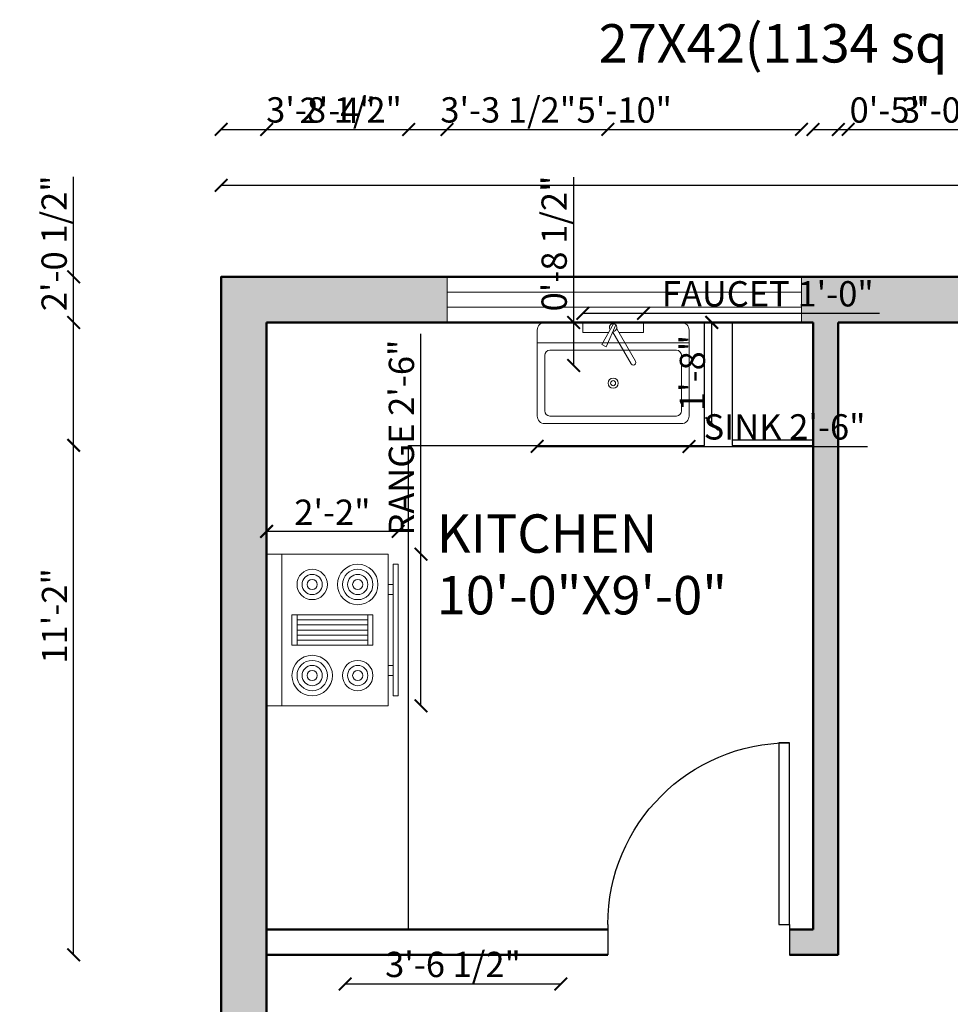
# Model space of a CAD drawing. Units: inches. Extents: x 1799 to 2247, y 1296 to 1881.
# Tile 3 of 4: x 1799 to 1983, y 1687 to 1881. Entities that reach past the tile are written whole.
import ezdxf

# ---------------------------------------------------------------- set-up
doc = ezdxf.new("R2010")
doc.units = ezdxf.units.IN
for name, color, linetype, lineweight in [('A-ANNO-DIMS', 2, 'Continuous', 18), ('A-ANNO-TEXT', 7, 'Continuous', 35), ('A-AREA-IDEN', 7, 'Continuous', 25), ('A-DOOR', 3, 'Continuous', 25), ('A-EQPM', 9, 'Continuous', 18), ('A-FLOR-CASE', 8, 'Continuous', 25), ('A-FLOR-FIXT', 9, 'Continuous', 18), ('A-WALL', 7, 'Continuous', 50), ('window', 4, 'Continuous', 18)]:
    doc.layers.add(name, color=color, linetype=linetype, lineweight=lineweight)
doc.layers.add('A-WALL-PATT', color=18, linetype='Continuous', lineweight=13, true_color=0x000000)
doc.styles.get("Standard").update_dxf_attribs({"font": 'arial.ttf'})
doc.dimstyles.new('ISO-25', dxfattribs={"dimtxt": 5, "dimasz": 2.5, "dimexe": 1.25, "dimexo": 0.625, "dimtad": 1, "dimdec": 0, "dimlunit": 4, "dimtxsty": 'Standard', "dimblk": 'ARCHTICK', "dimcen": 2.5, "dimse1": 1, "dimse2": 1, "dimclrd": 1, "dimadec": 0, "dimazin": 0, "dimtfac": 1, "dimtdec": 0, "dimtmove": 0, "dimatfit": 3, "dimfxl": 1, "dimarcsym": 0})

# ---------------------------------------------------------------- blocks, each defined once
blk = doc.blocks.new('Range-Oven - 30 in top')
for p, q in [((0, -3), (30, -3)), ((12, -6), (18, -6)), ((13, -20), (13, -6)), ((14, -6), (14, -20)), ((15, -20), (15, -6)), ((16, -6), (16, -20)), ((17, -20), (17, -6)), ((18, -20), (12, -20)), ((6, -24), (6, -25)), ((8, -25), (8, -24)), ((22, -25), (22, -24)), ((24, -24), (24, -25))]:
    blk.add_line(p, q)
for points in [[(0, -24), (0, 0), (30, 0), (30, -24)], [(12, -21), (12, -5), (18, -5), (18, -21)], [(2, -26), (2, -25), (28, -25), (28, -26)]]:
    blk.add_lwpolyline(points, close=True)
for centre, radius in [((6, -9), 4), ((6, -9), 3), ((6, -9), 2), ((24, -9), 3), ((24, -9), 2), ((6, -9), 1), ((24, -9), 1), ((6, -18), 3), ((24, -18), 4), ((24, -18), 3), ((6, -18), 2), ((6, -18), 1), ((24, -18), 2), ((24, -18), 1)]:
    blk.add_circle(centre, radius)
blk = doc.blocks.new('Faucet - single handle top')
for p, q in [((0.08, -0.26), (-2.26, -4.34)), ((-1.37, -4.79), (0.55, -0.5)), ((-0.06, -1.9), (3.57, -8.18)), ((4.43, -7.68), (0.72, -1.24)), ((-2.26, -4.34), (-1.37, -4.79))]:
    blk.add_line(p, q)
for points in [[(-0.92, -2), (-6, -2), (-6, 0), (6, 0), (6, -2), (1.16, -2)], [(-0.01, -2), (-0.12, -2)]]:
    blk.add_lwpolyline(points)
for centre, radius, start, end in [((0, -1), 0.75, 269.2246, 216.2304), ((4, -7.93), 0.5, 210, 30)]:
    blk.add_arc(centre, radius, start, end)
blk = doc.blocks.new('*U12')
for p, q in [((0, 0), (0, -5)), ((30, 0), (30, -5))]:
    blk.add_line(p, q)
blk.add_lwpolyline([(0, 0), (0, 30), (1.75, 30), (1.75, 0)], close=True)
blk.add_arc((0, 0), 30, 0, 90)
blk = doc.blocks.new('Sink-single - 30 in top')
blk.add_line((-15, -3.999996), (15, -3.999996))
for points in [[(-13.5, 0), (13.5, 0)], [(-15, -18.499996), (-15, -1.5)], [(15, -1.5), (15, -18.499996)], [(-12.5, -5.499996), (12.5, -5.499996)], [(-13.5, -17.499996), (-13.5, -6.499996)], [(13.5, -6.499996), (13.5, -17.499996)], [(12.5, -18.499996), (-12.5, -18.499996)], [(13.5, -19.999996), (-13.5, -19.999996)]]:
    blk.add_lwpolyline(points)
for radius in [1, 0.5]:
    blk.add_circle((0, -11.999996), radius)
for centre, radius, start, end in [((-13.5, -1.5), 1.5, 90, 180), ((13.5, -1.5), 1.5, 0, 90), ((-12.5, -6.499996), 1, 90, 180), ((12.5, -6.499996), 1, 0, 90), ((-12.5, -17.499996), 1, 180, 270), ((12.5, -17.499996), 1, 270, 0), ((-13.5, -18.499996), 1.5, 180, 270), ((13.5, -18.499996), 1.5, 270, 0)]:
    blk.add_arc(centre, radius, start, end)
blk = doc.blocks.new('_ArchTick')
at = {"color": 0, "linetype": 'ByBlock', "const_width": 0.15}
blk.add_lwpolyline([(-0.5, -0.5), (0.5, 0.5)], dxfattribs=at)
blk = doc.blocks.new('*D13')
at = {"layer": 'A-ANNO-DIMS', "color": 0, "lineweight": -2, "transparency": 16777216}
blk.add_line((1838.46, 1848.42), (2162.46, 1848.42), dxfattribs=at)
at = {"layer": 'Defpoints', "color": 0, "transparency": 16777216}
for p in [(2162.46, 1848.42), (1838.46, 1830.32), (2162.46, 1830.32)]:
    blk.add_point(p, dxfattribs=at)
at = {"layer": 'A-ANNO-DIMS', "color": 0, "lineweight": -2, "transparency": 16777216, "xscale": 2.5, "yscale": 2.5, "zscale": 2.5, "rotation": 180}
blk.add_blockref('_ArchTick', (1838.46, 1848.42), dxfattribs=at)
at = {"layer": 'A-ANNO-DIMS', "color": 0, "lineweight": -2, "transparency": 16777216, "xscale": 2.5, "yscale": 2.5, "zscale": 2.5}
blk.add_blockref('_ArchTick', (2162.46, 1848.42), dxfattribs=at)
at = {"layer": 'A-ANNO-DIMS', "color": 0, "transparency": 16777216, "insert": (2000.46, 1851.56), "char_height": 5, "attachment_point": 5}
blk.add_mtext("27'", dxfattribs=at)
blk = doc.blocks.new('*D23')
at = {"layer": 'A-ANNO-DIMS', "color": 1, "lineweight": -2, "transparency": 16777216}
blk.add_line((1862.99, 1690.58), (1905.61, 1690.58), dxfattribs=at)
at = {"layer": 'Defpoints', "color": 0, "transparency": 16777216}
for p in [(1905.61, 1690.58), (1862.99, 1680), (1905.61, 1680)]:
    blk.add_point(p, dxfattribs=at)
at = {"layer": 'A-ANNO-DIMS', "color": 1, "lineweight": -2, "transparency": 16777216, "xscale": 2.5, "yscale": 2.5, "zscale": 2.5, "rotation": 180}
blk.add_blockref('_ArchTick', (1862.99, 1690.58), dxfattribs=at)
at = {"layer": 'A-ANNO-DIMS', "color": 1, "lineweight": -2, "transparency": 16777216, "xscale": 2.5, "yscale": 2.5, "zscale": 2.5}
blk.add_blockref('_ArchTick', (1905.61, 1690.58), dxfattribs=at)
at = {"layer": 'A-ANNO-DIMS', "color": 0, "transparency": 16777216, "insert": (1884.3, 1693.79), "char_height": 5, "attachment_point": 5}
blk.add_mtext('3\'-6 1/2"', dxfattribs=at)
blk = doc.blocks.new('*D24')
at = {"layer": 'A-ANNO-DIMS', "color": 1, "lineweight": -2, "transparency": 16777216}
for p, q in [((1877.96, 1775.53), (1877.96, 1819.09)), ((1877.96, 1745.53), (1877.96, 1775.53))]:
    blk.add_line(p, q, dxfattribs=at)
at = {"layer": 'Defpoints', "color": 0, "transparency": 16777216}
for p in [(1873.46, 1775.53), (1877.96, 1775.53), (1873.46, 1745.53)]:
    blk.add_point(p, dxfattribs=at)
at = {"layer": 'A-ANNO-DIMS', "color": 1, "lineweight": -2, "transparency": 16777216, "xscale": 2.5, "yscale": 2.5, "zscale": 2.5}
for p, rotation in [((1877.96, 1775.53), 90), ((1877.96, 1745.53), 270)]:
    blk.add_blockref('_ArchTick', p, dxfattribs=dict(at, rotation=rotation))
at = {"layer": 'A-ANNO-DIMS', "color": 0, "transparency": 16777216, "insert": (1874.75, 1798.56), "char_height": 5, "attachment_point": 5, "rotation": 90}
blk.add_mtext('RANGE 2\'-6"', dxfattribs=at)
blk = doc.blocks.new('*D25')
at = {"layer": 'A-ANNO-DIMS', "color": 1, "lineweight": -2, "transparency": 16777216}
blk.add_line((1873.46, 1780.03), (1847.46, 1780.03), dxfattribs=at)
at = {"layer": 'Defpoints', "color": 0, "transparency": 16777216}
for p in [(1847.46, 1780.03), (1847.46, 1775.53), (1873.46, 1775.53)]:
    blk.add_point(p, dxfattribs=at)
at = {"layer": 'A-ANNO-DIMS', "color": 1, "lineweight": -2, "transparency": 16777216, "xscale": 2.5, "yscale": 2.5, "zscale": 2.5, "rotation": 180}
blk.add_blockref('_ArchTick', (1847.46, 1780.03), dxfattribs=at)
at = {"layer": 'A-ANNO-DIMS', "color": 1, "lineweight": -2, "transparency": 16777216, "xscale": 2.5, "yscale": 2.5, "zscale": 2.5}
blk.add_blockref('_ArchTick', (1873.46, 1780.03), dxfattribs=at)
at = {"layer": 'A-ANNO-DIMS', "color": 0, "transparency": 16777216, "insert": (1860.46, 1783.16), "char_height": 5, "attachment_point": 5}
blk.add_mtext('2\'-2"', dxfattribs=at)
blk = doc.blocks.new('*D26')
at = {"layer": 'A-ANNO-DIMS', "color": 1, "lineweight": -2, "transparency": 16777216}
for p, q in [((1900.95, 1796.82), (1930.95, 1796.82)), ((1930.95, 1796.82), (1966.21, 1796.82))]:
    blk.add_line(p, q, dxfattribs=at)
at = {"layer": 'Defpoints', "color": 0, "transparency": 16777216}
for p in [(1900.95, 1801.32), (1930.95, 1801.32), (1930.95, 1796.82)]:
    blk.add_point(p, dxfattribs=at)
at = {"layer": 'A-ANNO-DIMS', "color": 1, "lineweight": -2, "transparency": 16777216, "xscale": 2.5, "yscale": 2.5, "zscale": 2.5, "rotation": 180}
blk.add_blockref('_ArchTick', (1900.95, 1796.82), dxfattribs=at)
at = {"layer": 'A-ANNO-DIMS', "color": 1, "lineweight": -2, "transparency": 16777216, "xscale": 2.5, "yscale": 2.5, "zscale": 2.5}
blk.add_blockref('_ArchTick', (1930.95, 1796.82), dxfattribs=at)
at = {"layer": 'A-ANNO-DIMS', "color": 0, "transparency": 16777216, "insert": (1949.83, 1800.03), "char_height": 5, "attachment_point": 5}
blk.add_mtext('SINK 2\'-6"', dxfattribs=at)
blk = doc.blocks.new('*D27')
at = {"layer": 'A-ANNO-DIMS', "color": 1, "lineweight": -2, "transparency": 16777216}
blk.add_line((1935.45, 1801.32), (1935.45, 1821.32), dxfattribs=at)
at = {"layer": 'Defpoints', "color": 0, "transparency": 16777216}
for p in [(1930.95, 1821.32), (1935.45, 1821.32), (1930.95, 1801.32)]:
    blk.add_point(p, dxfattribs=at)
at = {"layer": 'A-ANNO-DIMS', "color": 1, "lineweight": -2, "transparency": 16777216, "xscale": 2.5, "yscale": 2.5, "zscale": 2.5}
for p, rotation in [((1935.45, 1821.32), 90), ((1935.45, 1801.32), 270)]:
    blk.add_blockref('_ArchTick', p, dxfattribs=dict(at, rotation=rotation))
at = {"layer": 'A-ANNO-DIMS', "color": 0, "transparency": 16777216, "insert": (1932.27, 1811.32), "char_height": 5, "attachment_point": 5, "rotation": 90}
blk.add_mtext('1\'-8"', dxfattribs=at)
blk = doc.blocks.new('*D28')
at = {"layer": 'A-ANNO-DIMS', "color": 1, "lineweight": -2, "transparency": 16777216}
for p, q in [((1909.95, 1823.12), (1921.95, 1823.12)), ((1921.95, 1823.12), (1968.59, 1823.12))]:
    blk.add_line(p, q, dxfattribs=at)
at = {"layer": 'Defpoints', "color": 0, "transparency": 16777216}
for p in [(1921.95, 1823.12), (1909.95, 1821.32), (1921.95, 1821.32)]:
    blk.add_point(p, dxfattribs=at)
at = {"layer": 'A-ANNO-DIMS', "color": 1, "lineweight": -2, "transparency": 16777216, "xscale": 2.5, "yscale": 2.5, "zscale": 2.5, "rotation": 180}
blk.add_blockref('_ArchTick', (1909.95, 1823.12), dxfattribs=at)
at = {"layer": 'A-ANNO-DIMS', "color": 1, "lineweight": -2, "transparency": 16777216, "xscale": 2.5, "yscale": 2.5, "zscale": 2.5}
blk.add_blockref('_ArchTick', (1921.95, 1823.12), dxfattribs=at)
at = {"layer": 'A-ANNO-DIMS', "color": 0, "transparency": 16777216, "insert": (1946.52, 1826.33), "char_height": 5, "attachment_point": 5}
blk.add_mtext('FAUCET 1\'-0"', dxfattribs=at)
blk = doc.blocks.new('*D29')
at = {"layer": 'A-ANNO-DIMS', "color": 1, "lineweight": -2, "transparency": 16777216}
for p, q in [((1908.15, 1821.32), (1908.15, 1850.01)), ((1908.15, 1812.82), (1908.15, 1821.32))]:
    blk.add_line(p, q, dxfattribs=at)
at = {"layer": 'Defpoints', "color": 0, "transparency": 16777216}
for p in [(1908.15, 1821.32), (1909.95, 1821.32), (1909.95, 1812.82)]:
    blk.add_point(p, dxfattribs=at)
at = {"layer": 'A-ANNO-DIMS', "color": 1, "lineweight": -2, "transparency": 16777216, "xscale": 2.5, "yscale": 2.5, "zscale": 2.5}
for p, rotation in [((1908.15, 1821.32), 90), ((1908.15, 1812.82), 270)]:
    blk.add_blockref('_ArchTick', p, dxfattribs=dict(at, rotation=rotation))
at = {"layer": 'A-ANNO-DIMS', "color": 0, "transparency": 16777216, "insert": (1904.94, 1836.92), "char_height": 5, "attachment_point": 5, "rotation": 90}
blk.add_mtext('0\'-8 1/2"', dxfattribs=at)
blk = doc.blocks.new('*D34')
at = {"layer": 'A-ANNO-DIMS', "color": 1, "lineweight": -2, "transparency": 16777216}
blk.add_line((1809.31, 1696.32), (1809.31, 1830.32), dxfattribs=at)
at = {"layer": 'Defpoints', "color": 0, "transparency": 16777216}
for p in [(1809.31, 1830.32), (1838.46, 1830.32), (1847.46, 1696.32)]:
    blk.add_point(p, dxfattribs=at)
at = {"layer": 'A-ANNO-DIMS', "color": 1, "lineweight": -2, "transparency": 16777216, "xscale": 2.5, "yscale": 2.5, "zscale": 2.5}
for p, rotation in [((1809.31, 1830.32), 90), ((1809.31, 1696.32), 270)]:
    blk.add_blockref('_ArchTick', p, dxfattribs=dict(at, rotation=rotation))
at = {"layer": 'A-ANNO-DIMS', "color": 0, "transparency": 16777216, "insert": (1806.17, 1763.32), "char_height": 5, "attachment_point": 5, "rotation": 90}
blk.add_mtext('11\'-2"', dxfattribs=at)
blk = doc.blocks.new('*D35')
at = {"layer": 'A-ANNO-DIMS', "color": 1, "lineweight": -2, "transparency": 16777216}
blk.add_line((1960.46, 1297.17), (2076.46, 1297.17), dxfattribs=at)
at = {"layer": 'Defpoints', "color": 0, "transparency": 16777216}
for p in [(1960.46, 1821.32), (2076.46, 1821.32), (2076.46, 1297.17)]:
    blk.add_point(p, dxfattribs=at)
at = {"layer": 'A-ANNO-DIMS', "color": 1, "lineweight": -2, "transparency": 16777216, "xscale": 2.5, "yscale": 2.5, "zscale": 2.5, "rotation": 180}
blk.add_blockref('_ArchTick', (1960.46, 1297.17), dxfattribs=at)
at = {"layer": 'A-ANNO-DIMS', "color": 1, "lineweight": -2, "transparency": 16777216, "xscale": 2.5, "yscale": 2.5, "zscale": 2.5}
blk.add_blockref('_ArchTick', (2076.46, 1297.17), dxfattribs=at)
at = {"layer": 'A-ANNO-DIMS', "color": 0, "transparency": 16777216, "insert": (2018.46, 1300.35), "char_height": 5, "attachment_point": 5}
blk.add_mtext('9\'-8"', dxfattribs=at)
blk = doc.blocks.new('*D36')
at = {"layer": 'A-ANNO-DIMS', "color": 1, "lineweight": -2, "transparency": 16777216}
blk.add_line((1847.46, 1859.47), (1875.53, 1859.47), dxfattribs=at)
at = {"layer": 'Defpoints', "color": 0, "transparency": 16777216}
for p in [(1875.53, 1859.47), (1847.46, 1701.32), (1875.53, 1701.32)]:
    blk.add_point(p, dxfattribs=at)
at = {"layer": 'A-ANNO-DIMS', "color": 1, "lineweight": -2, "transparency": 16777216, "xscale": 2.5, "yscale": 2.5, "zscale": 2.5, "rotation": 180}
blk.add_blockref('_ArchTick', (1847.46, 1859.47), dxfattribs=at)
at = {"layer": 'A-ANNO-DIMS', "color": 1, "lineweight": -2, "transparency": 16777216, "xscale": 2.5, "yscale": 2.5, "zscale": 2.5}
blk.add_blockref('_ArchTick', (1875.53, 1859.47), dxfattribs=at)
at = {"layer": 'A-ANNO-DIMS', "color": 0, "transparency": 16777216, "insert": (1861.5, 1862.6), "char_height": 5, "attachment_point": 5}
blk.add_mtext('2\'-4"', dxfattribs=at)
blk = doc.blocks.new('*D45')
at = {"layer": 'A-ANNO-DIMS', "color": 1, "lineweight": -2, "transparency": 16777216}
blk.add_line((1838.46, 1859.47), (1883.11, 1859.47), dxfattribs=at)
at = {"layer": 'Defpoints', "color": 0, "transparency": 16777216}
for p in [(1883.11, 1859.47), (1838.46, 1830.32), (1883.11, 1830.32)]:
    blk.add_point(p, dxfattribs=at)
at = {"layer": 'A-ANNO-DIMS', "color": 1, "lineweight": -2, "transparency": 16777216, "xscale": 2.5, "yscale": 2.5, "zscale": 2.5, "rotation": 180}
blk.add_blockref('_ArchTick', (1838.46, 1859.47), dxfattribs=at)
at = {"layer": 'A-ANNO-DIMS', "color": 1, "lineweight": -2, "transparency": 16777216, "xscale": 2.5, "yscale": 2.5, "zscale": 2.5}
blk.add_blockref('_ArchTick', (1883.11, 1859.47), dxfattribs=at)
at = {"layer": 'A-ANNO-DIMS', "color": 0, "transparency": 16777216, "insert": (1860.78, 1862.68), "char_height": 5, "attachment_point": 5}
blk.add_mtext('3\'-8 1/2"', dxfattribs=at)
blk = doc.blocks.new('*D46')
at = {"layer": 'A-ANNO-DIMS', "color": 1, "lineweight": -2, "transparency": 16777216}
blk.add_line((1883.11, 1859.47), (1953.2, 1859.47), dxfattribs=at)
at = {"layer": 'Defpoints', "color": 0, "transparency": 16777216}
for p in [(1953.2, 1859.47), (1883.11, 1830.32), (1953.2, 1830.32)]:
    blk.add_point(p, dxfattribs=at)
at = {"layer": 'A-ANNO-DIMS', "color": 1, "lineweight": -2, "transparency": 16777216, "xscale": 2.5, "yscale": 2.5, "zscale": 2.5, "rotation": 180}
blk.add_blockref('_ArchTick', (1883.11, 1859.47), dxfattribs=at)
at = {"layer": 'A-ANNO-DIMS', "color": 1, "lineweight": -2, "transparency": 16777216, "xscale": 2.5, "yscale": 2.5, "zscale": 2.5}
blk.add_blockref('_ArchTick', (1953.2, 1859.47), dxfattribs=at)
at = {"layer": 'A-ANNO-DIMS', "color": 0, "transparency": 16777216, "insert": (1918.16, 1862.65), "char_height": 5, "attachment_point": 5}
blk.add_mtext('5\'-10"', dxfattribs=at)
blk = doc.blocks.new('*D47')
at = {"layer": 'A-ANNO-DIMS', "color": 1, "lineweight": -2, "transparency": 16777216}
blk.add_line((1914.89, 1297.17), (1950.83, 1297.17), dxfattribs=at)
at = {"layer": 'Defpoints', "color": 0, "transparency": 16777216}
for p in [(1914.89, 1701.32), (1950.83, 1701.32), (1950.83, 1297.17)]:
    blk.add_point(p, dxfattribs=at)
at = {"layer": 'A-ANNO-DIMS', "color": 1, "lineweight": -2, "transparency": 16777216, "xscale": 2.5, "yscale": 2.5, "zscale": 2.5, "rotation": 180}
blk.add_blockref('_ArchTick', (1914.89, 1297.17), dxfattribs=at)
at = {"layer": 'A-ANNO-DIMS', "color": 1, "lineweight": -2, "transparency": 16777216, "xscale": 2.5, "yscale": 2.5, "zscale": 2.5}
blk.add_blockref('_ArchTick', (1950.83, 1297.17), dxfattribs=at)
at = {"layer": 'A-ANNO-DIMS', "color": 0, "transparency": 16777216, "insert": (1932.86, 1300.35), "char_height": 5, "attachment_point": 5}
blk.add_mtext('3\'-0"', dxfattribs=at)
blk = doc.blocks.new('*D48')
at = {"layer": 'A-ANNO-DIMS', "color": 1, "lineweight": -2, "transparency": 16777216}
blk.add_line((1962.42, 1859.47), (1998.36, 1859.47), dxfattribs=at)
at = {"layer": 'Defpoints', "color": 0, "transparency": 16777216}
for p in [(1998.36, 1859.47), (1962.42, 1353.51), (1998.36, 1353.51)]:
    blk.add_point(p, dxfattribs=at)
at = {"layer": 'A-ANNO-DIMS', "color": 1, "lineweight": -2, "transparency": 16777216, "xscale": 2.5, "yscale": 2.5, "zscale": 2.5, "rotation": 180}
blk.add_blockref('_ArchTick', (1962.42, 1859.47), dxfattribs=at)
at = {"layer": 'A-ANNO-DIMS', "color": 1, "lineweight": -2, "transparency": 16777216, "xscale": 2.5, "yscale": 2.5, "zscale": 2.5}
blk.add_blockref('_ArchTick', (1998.36, 1859.47), dxfattribs=at)
at = {"layer": 'A-ANNO-DIMS', "color": 0, "transparency": 16777216, "insert": (1980.39, 1862.65), "char_height": 5, "attachment_point": 5}
blk.add_mtext('3\'-0"', dxfattribs=at)
blk = doc.blocks.new('*D55')
at = {"layer": 'A-ANNO-DIMS', "color": 1, "lineweight": -2, "transparency": 16777216}
blk.add_line((2242.61, 1701.32), (2242.61, 1745.53), dxfattribs=at)
at = {"layer": 'Defpoints', "color": 0, "transparency": 16777216}
for p in [(1847.46, 1745.53), (2242.61, 1745.53), (1847.46, 1701.32)]:
    blk.add_point(p, dxfattribs=at)
at = {"layer": 'A-ANNO-DIMS', "color": 1, "lineweight": -2, "transparency": 16777216, "xscale": 2.5, "yscale": 2.5, "zscale": 2.5}
for p, rotation in [((2242.61, 1745.53), 90), ((2242.61, 1701.32), 270)]:
    blk.add_blockref('_ArchTick', p, dxfattribs=dict(at, rotation=rotation))
at = {"layer": 'A-ANNO-DIMS', "color": 0, "transparency": 16777216, "insert": (2239.43, 1723.42), "char_height": 5, "attachment_point": 5, "rotation": 90}
blk.add_mtext('3\'-8"', dxfattribs=at)
blk = doc.blocks.new('*D56')
at = {"layer": 'A-ANNO-DIMS', "color": 1, "lineweight": -2, "transparency": 16777216}
for p, q in [((1809.31, 1821.32), (1809.31, 1850.1)), ((1809.31, 1797.03), (1809.31, 1821.32))]:
    blk.add_line(p, q, dxfattribs=at)
at = {"layer": 'Defpoints', "color": 0, "transparency": 16777216}
for p in [(1809.31, 1821.32), (1955.46, 1821.32), (1955.46, 1797.03)]:
    blk.add_point(p, dxfattribs=at)
at = {"layer": 'A-ANNO-DIMS', "color": 1, "lineweight": -2, "transparency": 16777216, "xscale": 2.5, "yscale": 2.5, "zscale": 2.5}
for p, rotation in [((1809.31, 1821.32), 90), ((1809.31, 1797.03), 270)]:
    blk.add_blockref('_ArchTick', p, dxfattribs=dict(at, rotation=rotation))
at = {"layer": 'A-ANNO-DIMS', "color": 0, "transparency": 16777216, "insert": (1806.1, 1836.96), "char_height": 5, "attachment_point": 5, "rotation": 90}
blk.add_mtext('2\'-0 1/2"', dxfattribs=at)
blk = doc.blocks.new('*D57')
at = {"layer": 'A-ANNO-DIMS', "color": 1, "lineweight": -2, "transparency": 16777216}
blk.add_line((1875.53, 1297.17), (1901.39, 1297.17), dxfattribs=at)
at = {"layer": 'Defpoints', "color": 0, "transparency": 16777216}
for p in [(1901.39, 1801.76), (1875.53, 1797.03), (1901.39, 1297.17)]:
    blk.add_point(p, dxfattribs=at)
at = {"layer": 'A-ANNO-DIMS', "color": 1, "lineweight": -2, "transparency": 16777216, "xscale": 2.5, "yscale": 2.5, "zscale": 2.5, "rotation": 180}
blk.add_blockref('_ArchTick', (1875.53, 1297.17), dxfattribs=at)
at = {"layer": 'A-ANNO-DIMS', "color": 1, "lineweight": -2, "transparency": 16777216, "xscale": 2.5, "yscale": 2.5, "zscale": 2.5}
blk.add_blockref('_ArchTick', (1901.39, 1297.17), dxfattribs=at)
at = {"layer": 'A-ANNO-DIMS', "color": 0, "transparency": 16777216, "insert": (1888.46, 1300.3), "char_height": 5, "attachment_point": 5}
blk.add_mtext('2\'-2"', dxfattribs=at)
blk = doc.blocks.new('*D61')
at = {"layer": 'A-ANNO-DIMS', "color": 1, "lineweight": -2, "transparency": 16777216}
for p, q in [((1838.46, 1297.17), (1847.46, 1297.17)), ((1847.46, 1297.17), (1864.5, 1297.17))]:
    blk.add_line(p, q, dxfattribs=at)
at = {"layer": 'Defpoints', "color": 0, "transparency": 16777216}
for p in [(1838.46, 1830.32), (1847.46, 1821.32), (1847.46, 1297.17)]:
    blk.add_point(p, dxfattribs=at)
at = {"layer": 'A-ANNO-DIMS', "color": 1, "lineweight": -2, "transparency": 16777216, "xscale": 2.5, "yscale": 2.5, "zscale": 2.5, "rotation": 180}
blk.add_blockref('_ArchTick', (1838.46, 1297.17), dxfattribs=at)
at = {"layer": 'A-ANNO-DIMS', "color": 1, "lineweight": -2, "transparency": 16777216, "xscale": 2.5, "yscale": 2.5, "zscale": 2.5}
blk.add_blockref('_ArchTick', (1847.46, 1297.17), dxfattribs=at)
at = {"layer": 'A-ANNO-DIMS', "color": 0, "transparency": 16777216, "insert": (1857.23, 1300.35), "char_height": 5, "attachment_point": 5}
blk.add_mtext('0\'-9"', dxfattribs=at)
blk = doc.blocks.new('*D62')
at = {"layer": 'A-ANNO-DIMS', "color": 1, "lineweight": -2, "transparency": 16777216}
for p, q in [((1955.46, 1859.47), (1960.46, 1859.47)), ((1960.46, 1859.47), (1977.5, 1859.47))]:
    blk.add_line(p, q, dxfattribs=at)
at = {"layer": 'Defpoints', "color": 0, "transparency": 16777216}
for p in [(1960.46, 1859.47), (1955.46, 1821.32), (1960.46, 1821.32)]:
    blk.add_point(p, dxfattribs=at)
at = {"layer": 'A-ANNO-DIMS', "color": 1, "lineweight": -2, "transparency": 16777216, "xscale": 2.5, "yscale": 2.5, "zscale": 2.5, "rotation": 180}
blk.add_blockref('_ArchTick', (1955.46, 1859.47), dxfattribs=at)
at = {"layer": 'A-ANNO-DIMS', "color": 1, "lineweight": -2, "transparency": 16777216, "xscale": 2.5, "yscale": 2.5, "zscale": 2.5}
blk.add_blockref('_ArchTick', (1960.46, 1859.47), dxfattribs=at)
at = {"layer": 'A-ANNO-DIMS', "color": 0, "transparency": 16777216, "insert": (1970.23, 1862.65), "char_height": 5, "attachment_point": 5}
blk.add_mtext('0\'-5"', dxfattribs=at)
blk = doc.blocks.new('*D63')
at = {"layer": 'A-ANNO-DIMS', "color": 1, "lineweight": -2, "transparency": 16777216}
blk.add_line((1875.53, 1859.47), (1914.89, 1859.47), dxfattribs=at)
at = {"layer": 'Defpoints', "color": 0, "transparency": 16777216}
for p in [(1914.89, 1859.47), (1875.53, 1701.32), (1914.89, 1701.32)]:
    blk.add_point(p, dxfattribs=at)
at = {"layer": 'A-ANNO-DIMS', "color": 1, "lineweight": -2, "transparency": 16777216, "xscale": 2.5, "yscale": 2.5, "zscale": 2.5, "rotation": 180}
blk.add_blockref('_ArchTick', (1875.53, 1859.47), dxfattribs=at)
at = {"layer": 'A-ANNO-DIMS', "color": 1, "lineweight": -2, "transparency": 16777216, "xscale": 2.5, "yscale": 2.5, "zscale": 2.5}
blk.add_blockref('_ArchTick', (1914.89, 1859.47), dxfattribs=at)
at = {"layer": 'A-ANNO-DIMS', "color": 0, "transparency": 16777216, "insert": (1895.21, 1862.68), "char_height": 5, "attachment_point": 5}
blk.add_mtext('3\'-3 1/2"', dxfattribs=at)

msp = doc.modelspace()

# ---------------------------------------------------------------- hatches: boundary and pattern name
at = {"layer": 'A-WALL-PATT'}
h = msp.add_hatch(color=256, dxfattribs=at)
h.dxf.hatch_style = 1
h.paths.add_polyline_path([(1847.46, 1821.32), (1883.11, 1821.32), (1883.11, 1830.32), (1838.46, 1830.32), (1838.46, 1618.8), (1847.46, 1618.8)])
h.paths.add_polyline_path([(1847.46, 1534.31), (1838.46, 1534.31), (1838.46, 1444.97), (1847.46, 1444.97)])
h.paths.add_polyline_path([(1847.46, 1404.13), (1838.46, 1404.13), (1838.46, 1353.51), (1847.46, 1353.51), (1962.42, 1353.51), (1962.42, 1359.5, -0.020971), (1962.55, 1362.51), (1847.46, 1362.51)])
h.paths.add_polyline_path([(2162.46, 1509.73), (2153.46, 1509.73), (2153.46, 1493.32), (2075.46, 1493.32), (2075.46, 1496.56), (2075.02, 1496.56), (2070.46, 1496.56), (2070.46, 1488.32), (2153.46, 1488.32), (2153.46, 1335.32), (2119.37, 1335.32), (2119.37, 1326.32), (2162.46, 1326.32)])
h.paths.add_polyline_path([(2059.58, 1335.32), (2008.46, 1335.32), (2008.46, 1353.51), (2003.46, 1353.51), (2003.46, 1335.32), (2003.46, 1326.32), (2059.58, 1326.32)])
h.paths.add_polyline_path([(2008.46, 1471.58), (2003.46, 1471.58), (2003.46, 1460.32), (1847.46, 1460.32), (1847.46, 1455.32), (2003.46, 1455.32), (2003.46, 1362.51), (2008.46, 1362.51)])
h.paths.add_polyline_path([(2008.46, 1362.51), (2003.46, 1362.51), (2003.46, 1353.51), (2008.46, 1353.51)])
h.paths.add_polyline_path([(2003.46, 1362.51), (1998.36, 1362.51), (1998.36, 1359.5), (1998.36, 1353.51), (2003.46, 1353.51)])
h.paths.add_polyline_path([(1989.49, 1830.32), (1953.2, 1830.32), (1953.2, 1821.32), (1955.46, 1821.32), (1955.46, 1701.32), (1950.83, 1701.32), (1950.83, 1696.32), (1960.46, 1696.32), (1960.46, 1821.32), (1989.49, 1821.32)])
h.paths.add_polyline_path([(2162.46, 1606.83), (2153.46, 1606.83), (2153.46, 1541.93), (2162.46, 1541.93)])
h.paths.add_polyline_path([(2162.46, 1746.71), (2153.46, 1746.71), (2153.46, 1701.32), (2081.46, 1701.32), (2081.46, 1707.91), (2081.05, 1707.91), (2076.46, 1707.91), (2076.46, 1701.32), (2003.46, 1701.32), (2003.46, 1604.81), (2008.46, 1604.81), (2008.46, 1696.32), (2153.46, 1696.32), (2153.46, 1656.83), (2162.46, 1656.83)])
h.paths.add_polyline_path([(2162.46, 1830.32), (2050.89, 1830.32), (2050.89, 1821.32), (2076.46, 1821.32), (2076.46, 1735.44), (2081.05, 1735.44, -0.003736), (2081.46, 1735.44), (2081.46, 1821.32), (2153.46, 1821.32), (2153.46, 1778.8), (2162.46, 1778.8)])
h.paths.add_polyline_path([(1961.29, 1344.27), (2000.99, 1344.27), (2000.99, 1355.65), (1961.29, 1355.65)], flags=9)
h.paths.add_polyline_path([(1882.83, 1491.06), (1947.74, 1491.06), (1947.74, 1502.69), (1882.83, 1502.69)], flags=9)
h.paths.add_polyline_path([(1882.8, 1503.23), (1950.9, 1503.23), (1950.9, 1514.99), (1882.8, 1514.99)], flags=9)
h.paths.add_polyline_path([(2045.91, 1444.14), (2110.82, 1444.14), (2110.82, 1455.75), (2045.91, 1455.75)], flags=9)
h.paths.add_polyline_path([(2045.88, 1456.29), (2116.91, 1456.29), (2116.91, 1468.06), (2045.88, 1468.06)], flags=9)
h.paths.add_polyline_path([(2084.43, 1526.38), (2124.38, 1526.38), (2124.38, 1537.99), (2084.43, 1537.99)], flags=9)
h.paths.add_polyline_path([(2084.4, 1538.53), (2125.41, 1538.53), (2125.41, 1550.3), (2084.4, 1550.3)], flags=9)
h.paths.add_polyline_path([(2013.59, 1530.05), (2066.72, 1530.05), (2066.72, 1541.67), (2013.59, 1541.67)], flags=9)
h.paths.add_polyline_path([(2013.56, 1542.21), (2053.98, 1542.21), (2053.98, 1553.97), (2013.56, 1553.97)], flags=9)
h.paths.add_polyline_path([(2054.17, 1583.99), (2119.08, 1583.99), (2119.08, 1595.62), (2054.17, 1595.62)], flags=9)
h.paths.add_polyline_path([(2054.14, 1596.16), (2125.17, 1596.16), (2125.17, 1607.93), (2054.14, 1607.93)], flags=9)
h.paths.add_polyline_path([(2091.32, 1783.78), (2144.45, 1783.78), (2144.45, 1795.39), (2091.32, 1795.39)], flags=25)
h.paths.add_polyline_path([(2091.3, 1795.93), (2142.9, 1795.93), (2142.9, 1807.7), (2091.3, 1807.7)], flags=25)
h.paths.add_polyline_path([(1985.13, 1779.5), (2017.8, 1779.5), (2017.8, 1790.88), (1985.13, 1790.88)], flags=9)
h.paths.add_polyline_path([(1985.08, 1791.49), (2020.79, 1791.49), (2020.79, 1803.25), (1985.08, 1803.25)], flags=9)
h.paths.add_polyline_path([(1879.15, 1761.55), (1938.17, 1761.55), (1938.17, 1773.17), (1879.15, 1773.17)], flags=9)
h.paths.add_polyline_path([(1879.13, 1773.71), (1929.55, 1773.71), (1929.55, 1785.47), (1879.13, 1785.47)], flags=9)

# ---------------------------------------------------------------- linework, layer by layer
at = {"layer": 'A-FLOR-CASE'}
for p, q in [((1934.01, 1797.03), (1934.01, 1821.32)), ((1939.46, 1821.32), (1939.46, 1797.03)), ((1939.46, 1798.13), (1955.46, 1798.13)), ((1875.53, 1701.32), (1875.53, 1797.03)), ((1875.53, 1797.03), (1934.01, 1797.03)), ((1939.46, 1797.03), (1955.46, 1797.03))]:
    msp.add_line(p, q, dxfattribs=at)
at = {"layer": 'A-WALL'}
for p, q in [((1847.46, 1821.32), (1955.46, 1821.32)), ((1847.46, 1362.51), (1847.46, 1821.32)), ((1955.46, 1701.32), (1955.46, 1821.32)), ((1960.46, 1696.32), (1960.46, 1821.32)), ((1960.46, 1821.32), (2076.46, 1821.32)), ((1847.46, 1701.32), (1914.89, 1701.32)), ((1950.83, 1701.32), (1955.46, 1701.32)), ((1847.46, 1696.32), (1914.89, 1696.32)), ((1950.83, 1696.32), (1960.46, 1696.32))]:
    msp.add_line(p, q, dxfattribs=at)
msp.add_lwpolyline([(1838.46, 1353.51), (1838.46, 1830.32), (2162.46, 1830.32), (2162.46, 1326.32), (2003.46, 1326.32)], dxfattribs=at)
at = {"layer": 'window'}
for p, q in [((1883.11, 1821.32), (1883.11, 1830.32)), ((1883.11, 1830.32), (1953.2, 1830.32)), ((1953.2, 1830.32), (1953.2, 1821.32)), ((1883.11, 1827.32), (1953.2, 1827.32)), ((1883.11, 1824.32), (1953.2, 1824.32)), ((1953.2, 1821.32), (1883.11, 1821.32))]:
    msp.add_line(p, q, dxfattribs=at)

# ---------------------------------------------------------------- block references
at = {"layer": 'A-DOOR', "xscale": -1.197883670562129, "yscale": 1.197883670562129, "zscale": 1.197883670562129}
msp.add_blockref('*U12', (1950.83, 1702.31), dxfattribs=at)
at = {"layer": 'A-EQPM', "rotation": 90}
msp.add_blockref('Range-Oven - 30 in top', (1847.46, 1745.53), dxfattribs=at)
at = {"layer": 'A-FLOR-FIXT'}
for name in ['Sink-single - 30 in top', 'Faucet - single handle top']:
    msp.add_blockref(name, (1915.95, 1821.32), dxfattribs=at)

# ---------------------------------------------------------------- texts
at = {"layer": 'A-ANNO-TEXT'}
msp.add_text('27X42(1134 sq ft) house plan-North face', height=7.5834, dxfattribs=at).set_placement((1913.09, 1872.69))
at = {"layer": 'A-AREA-IDEN'}
for s, height, p in [('KITCHEN', 7.583, (1881.09, 1775.8)), ('10\'-0"X9\'-0"', 7.5834, (1881.09, 1763.62))]:
    msp.add_text(s, height=height, dxfattribs=at).set_placement(p)

# ---------------------------------------------------------------- dimensions: what is measured, and where the dimension line sits
at = {"layer": 'A-ANNO-DIMS'}
for base, p1, p2, override, picture, middle in [((1883.1123, 1859.469), (1838.4567, 1830.319), (1883.1123, 1830.319), {"dimdec": 1, "dimlfac": 1, "dimrnd": 0, "dimzin": 1, "dimdsep": 46, "dimlunit": 4, "dimfrac": 2}, '*D45', (1860.7845, 1862.681)), ((1914.89, 1859.47), (1875.53, 1701.32), (1914.89, 1701.32), {"dimdec": 1, "dimlfac": 1, "dimrnd": 0, "dimzin": 1, "dimdsep": 46, "dimlunit": 4, "dimfrac": 2}, '*D63', (1895.21, 1862.68)), ((1875.53, 1859.47), (1847.46, 1701.32), (1875.53, 1701.32), {"dimdec": 1, "dimlfac": 1, "dimrnd": 0, "dimzin": 1, "dimdsep": 46, "dimlunit": 4, "dimfrac": 2}, '*D36', (1861.5, 1862.6)), ((1953.2, 1859.47), (1883.11, 1830.32), (1953.2, 1830.32), {"dimdec": 1, "dimlfac": 1, "dimrnd": 0, "dimzin": 1, "dimdsep": 46, "dimlunit": 4, "dimfrac": 2}, '*D46', (1918.16, 1862.65)), ((1960.46, 1859.47), (1955.46, 1821.32), (1960.46, 1821.32), {"dimdec": 1, "dimlfac": 1, "dimrnd": 0, "dimzin": 1, "dimdsep": 46, "dimlunit": 4, "dimfrac": 2}, '*D62', (1970.23, 1862.65)), ((1998.36, 1859.47), (1962.42, 1353.51), (1998.36, 1353.51), {"dimdec": 1, "dimlfac": 1, "dimrnd": 0, "dimzin": 1, "dimdsep": 46, "dimlunit": 4, "dimfrac": 2}, '*D48', (1980.39, 1862.65)), ((2162.46, 1848.42), (1838.46, 1830.32), (2162.46, 1830.32), {"dimclrd": 0, "dimclre": 0, "dimclrt": 0}, '*D13', (2000.46, 1851.56)), ((1847.46, 1297.17), (1838.46, 1830.32), (1847.46, 1821.32), {"dimdec": 1, "dimlfac": 1, "dimrnd": 0, "dimzin": 1, "dimdsep": 46, "dimlunit": 4, "dimfrac": 2}, '*D61', (1857.23, 1300.35)), ((2076.46, 1297.17), (1960.46, 1821.32), (2076.46, 1821.32), {"dimdec": 1, "dimlfac": 1, "dimrnd": 0, "dimzin": 1, "dimdsep": 46, "dimlunit": 4, "dimfrac": 2}, '*D35', (2018.46, 1300.35)), ((1901.39, 1297.17), (1875.53, 1797.03), (1901.39, 1801.76), {"dimdec": 1, "dimlfac": 1, "dimrnd": 0, "dimzin": 1, "dimdsep": 46, "dimlunit": 4, "dimfrac": 2}, '*D57', (1888.46, 1300.3)), ((1905.61, 1690.58), (1862.99, 1680), (1905.61, 1680), {"dimdec": 1, "dimlfac": 1, "dimrnd": 0, "dimzin": 1, "dimdsep": 46, "dimlunit": 4, "dimfrac": 2}, '*D23', (1884.3, 1693.79)), ((1950.83, 1297.17), (1914.89, 1701.32), (1950.83, 1701.32), {"dimdec": 1, "dimlfac": 1, "dimrnd": 0, "dimzin": 1, "dimdsep": 46, "dimlunit": 4, "dimfrac": 2}, '*D47', (1932.86, 1300.35))]:
    dim = msp.add_linear_dim(base=base, p1=p1, p2=p2, dimstyle='ISO-25', override=override, dxfattribs=at)
    dim.commit()
    dim.dimension.update_dxf_attribs({"geometry": picture, "text_midpoint": middle})
for base, p1, p2, angle, picture, middle in [((1809.31, 1821.32), (1955.46, 1797.03), (1955.46, 1821.32), 90, '*D56', (1806.1, 1836.96)), ((1908.15, 1821.32), (1909.95, 1812.82), (1909.95, 1821.32), 90, '*D29', (1904.94, 1836.92)), ((1809.31, 1830.32), (1847.46, 1696.32), (1838.46, 1830.32), 90, '*D34', (1806.17, 1763.32)), ((1935.45, 1821.32), (1930.95, 1801.32), (1930.95, 1821.32), 90, '*D27', (1932.27, 1811.32)), ((1847.46, 1780.03), (1873.46, 1775.53), (1847.46, 1775.53), 180, '*D25', (1860.46, 1783.16)), ((2242.61, 1745.53), (1847.46, 1701.32), (1847.46, 1745.53), 90, '*D55', (2239.43, 1723.42))]:
    dim = msp.add_linear_dim(base=base, p1=p1, p2=p2, angle=angle, dimstyle='ISO-25', override={"dimdec": 1, "dimlfac": 1, "dimrnd": 0, "dimzin": 1, "dimdsep": 46, "dimlunit": 4, "dimfrac": 2}, dxfattribs=at)
    dim.commit()
    dim.dimension.update_dxf_attribs({"geometry": picture, "text_midpoint": middle})
for base, p1, p2, text, picture, middle in [((1921.95, 1823.12), (1909.95, 1821.32), (1921.95, 1821.32), 'FAUCET <>', '*D28', (1946.52, 1826.33)), ((1930.95, 1796.82), (1900.95, 1801.32), (1930.95, 1801.32), 'SINK <>', '*D26', (1949.83, 1800.03))]:
    dim = msp.add_linear_dim(base=base, p1=p1, p2=p2, text=text, dimstyle='ISO-25', override={"dimdec": 1, "dimlfac": 1, "dimrnd": 0, "dimzin": 1, "dimdsep": 46, "dimlunit": 4, "dimfrac": 2}, dxfattribs=at)
    dim.commit()
    dim.dimension.update_dxf_attribs({"geometry": picture, "text_midpoint": middle})
dim = msp.add_linear_dim(base=(1877.96, 1775.53), p1=(1873.46, 1745.53), p2=(1873.46, 1775.53), angle=90, text='RANGE <>', dimstyle='ISO-25', override={"dimdec": 1, "dimlfac": 1, "dimrnd": 0, "dimzin": 1, "dimdsep": 46, "dimlunit": 4, "dimfrac": 2}, dxfattribs=at)
dim.commit()
dim.dimension.update_dxf_attribs({"geometry": '*D24', "text_midpoint": (1874.75, 1798.56)})

doc.saveas('drawing.dxf')
